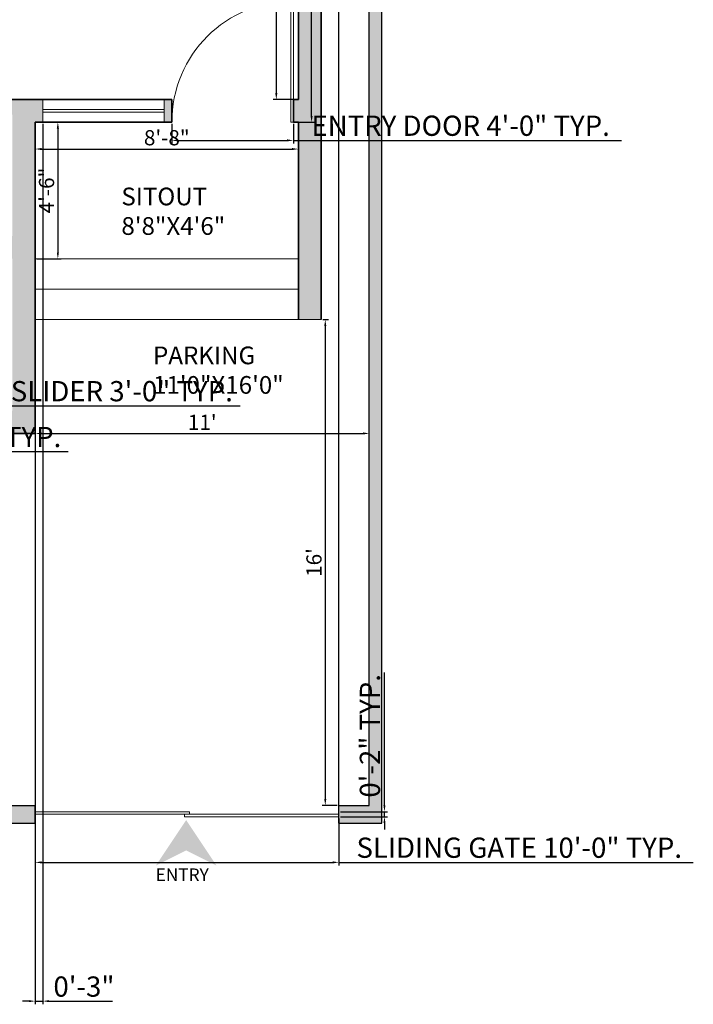
# Model space of a CAD drawing. Units: inches. Extents: x 2700 to 4052, y 1030 to 1872.
# Tile 6 of 8: x 3786 to 4052, y 1030 to 1419. Entities that reach past the tile are written whole.
import ezdxf

# ---------------------------------------------------------------- set-up
doc = ezdxf.new("R2010")
doc.units = ezdxf.units.IN
for name, color, linetype, lineweight in [('A-ANNO-DIMS', 2, 'Continuous', 13), ('A-ANNO-SYMB', 7, 'Continuous', 18), ('A-ANNO-TEXT', 7, 'Continuous', 18), ('A-AREA-IDEN', 7, 'Continuous', 18), ('A-DOOR', 4, 'Continuous', 18), ('A-FLOR-STRS', 7, 'Continuous', 18), ('A-GLAZ', 4, 'Continuous', 18), ('A-WALL', 7, 'Continuous', 35), ('A-WALL-PATT', 7, 'Continuous', 13), ('C-PROP', 7, 'Continuous', 25), ('C-SITE-GATE', 7, 'Continuous', 18)]:
    doc.layers.add(name, color=color, linetype=linetype, lineweight=lineweight)
doc.layers.add('C-SITE-PATT', color=252, linetype='Continuous', lineweight=13, true_color=0x939598)
doc.styles.get("Standard").update_dxf_attribs({"font": 'arial.ttf'})
doc.dimstyles.new('ISO-25', dxfattribs={"dimtxt": 8, "dimasz": 2.5, "dimexe": 1.25, "dimexo": 0.625, "dimtad": 1, "dimdec": 1, "dimlunit": 3, "dimtxsty": 'Standard', "dimcen": 2.5, "dimclrt": 1, "dimadec": 0, "dimazin": 0, "dimtfac": 1, "dimtdec": 1, "dimtmove": 0, "dimatfit": 3, "dimfxl": 1, "dimarcsym": 0})

# ---------------------------------------------------------------- blocks, each defined once
blk = doc.blocks.new('*D49')
at = {"layer": 'A-ANNO-DIMS', "color": 0, "lineweight": -2, "transparency": 16777216}
for p, q in [((3895.26, 1627.52), (3885.9, 1627.52)), ((3887.15, 1625.02), (3887.15, 1390.02)), ((3895.26, 1387.52), (3885.9, 1387.52))]:
    blk.add_line(p, q, dxfattribs=at)
at = {"layer": 'A-ANNO-DIMS', "color": 0, "transparency": 16777216}
for points in [[(3886.73, 1625.02), (3887.57, 1625.02), (3887.15, 1627.52)], [(3886.73, 1390.02), (3887.57, 1390.02), (3887.15, 1387.52)]]:
    blk.add_solid(points, dxfattribs=at)
at = {"layer": 'Defpoints', "color": 0, "transparency": 16777216}
for p in [(3895.88, 1627.52), (3887.15, 1387.52), (3895.88, 1387.52)]:
    blk.add_point(p, dxfattribs=at)
at = {"layer": 'A-ANNO-DIMS', "color": 0, "transparency": 16777216, "insert": (3883.46, 1507.52), "char_height": 6, "attachment_point": 5, "rotation": 90}
blk.add_mtext("20'", dxfattribs=at)
blk = doc.blocks.new('*D50')
at = {"layer": 'A-ANNO-DIMS', "color": 0, "lineweight": -2, "transparency": 16777216}
for p, q in [((3792.51, 1378.52), (3802.08, 1378.52)), ((3800.83, 1376.02), (3800.83, 1327.02)), ((3792.51, 1324.52), (3802.08, 1324.52))]:
    blk.add_line(p, q, dxfattribs=at)
at = {"layer": 'A-ANNO-DIMS', "color": 0, "transparency": 16777216}
for points in [[(3800.41, 1376.02), (3801.24, 1376.02), (3800.83, 1378.52)], [(3800.41, 1327.02), (3801.24, 1327.02), (3800.83, 1324.52)]]:
    blk.add_solid(points, dxfattribs=at)
at = {"layer": 'Defpoints', "color": 0, "transparency": 16777216}
for p in [(3791.88, 1378.52), (3791.88, 1324.52), (3800.83, 1324.52)]:
    blk.add_point(p, dxfattribs=at)
at = {"layer": 'A-ANNO-DIMS', "color": 0, "transparency": 16777216, "insert": (3797.14, 1351.52), "char_height": 6, "attachment_point": 5, "rotation": 90}
blk.add_mtext('4\'-6"', dxfattribs=at)
blk = doc.blocks.new('*D51')
at = {"layer": 'A-ANNO-DIMS', "color": 0, "lineweight": -2, "transparency": 16777216}
for p, q in [((3791.88, 1377.89), (3791.88, 1366.65)), ((3895.88, 1377.89), (3895.88, 1366.65)), ((3794.38, 1367.9), (3893.38, 1367.9))]:
    blk.add_line(p, q, dxfattribs=at)
at = {"layer": 'A-ANNO-DIMS', "color": 0, "transparency": 16777216}
for points in [[(3794.38, 1368.32), (3794.38, 1367.49), (3791.88, 1367.9)], [(3893.38, 1368.32), (3893.38, 1367.49), (3895.88, 1367.9)]]:
    blk.add_solid(points, dxfattribs=at)
at = {"layer": 'Defpoints', "color": 0, "transparency": 16777216}
for p in [(3791.88, 1378.52), (3895.88, 1378.52), (3895.88, 1367.9)]:
    blk.add_point(p, dxfattribs=at)
at = {"layer": 'A-ANNO-DIMS', "color": 0, "transparency": 16777216, "insert": (3843.88, 1371.59), "char_height": 6, "attachment_point": 5}
blk.add_mtext('8\'-8"', dxfattribs=at)
blk = doc.blocks.new('*D52')
at = {"layer": 'A-ANNO-DIMS', "color": 0, "lineweight": -2, "transparency": 16777216}
for p, q in [((3791.88, 1256.14), (3791.88, 1256.77)), ((3923.88, 1256.14), (3923.88, 1256.77)), ((3794.38, 1255.52), (3921.38, 1255.52))]:
    blk.add_line(p, q, dxfattribs=at)
at = {"layer": 'A-ANNO-DIMS', "color": 0, "transparency": 16777216}
for points in [[(3794.38, 1255.93), (3794.38, 1255.1), (3791.88, 1255.52)], [(3921.38, 1255.93), (3921.38, 1255.1), (3923.88, 1255.52)]]:
    blk.add_solid(points, dxfattribs=at)
at = {"layer": 'Defpoints', "color": 0, "transparency": 16777216}
for p in [(3791.88, 1255.52), (3923.88, 1255.52), (3923.88, 1255.52)]:
    blk.add_point(p, dxfattribs=at)
at = {"layer": 'A-ANNO-DIMS', "color": 0, "transparency": 16777216, "insert": (3857.88, 1259.15), "char_height": 6, "attachment_point": 5}
blk.add_mtext("11'", dxfattribs=at)
blk = doc.blocks.new('*D53')
at = {"layer": 'A-ANNO-DIMS', "color": 0, "lineweight": -2, "transparency": 16777216}
for p, q in [((3905.51, 1300.52), (3907.75, 1300.52)), ((3906.5, 1298.02), (3906.5, 1111.02)), ((3911.26, 1108.52), (3905.25, 1108.52))]:
    blk.add_line(p, q, dxfattribs=at)
at = {"layer": 'A-ANNO-DIMS', "color": 0, "transparency": 16777216}
for points in [[(3906.09, 1298.02), (3906.92, 1298.02), (3906.5, 1300.52)], [(3906.09, 1111.02), (3906.92, 1111.02), (3906.5, 1108.52)]]:
    blk.add_solid(points, dxfattribs=at)
at = {"layer": 'Defpoints', "color": 0, "transparency": 16777216}
for p in [(3904.88, 1300.52), (3906.5, 1108.52), (3911.88, 1108.52)]:
    blk.add_point(p, dxfattribs=at)
at = {"layer": 'A-ANNO-DIMS', "color": 0, "transparency": 16777216, "insert": (3902.81, 1204.52), "char_height": 6, "attachment_point": 5, "rotation": 90}
blk.add_mtext("16'", dxfattribs=at)
blk = doc.blocks.new('DOOR-SWING-48IN')
for p, q in [((-1, 48), (-1, 0)), ((0, 48), (0, 0)), ((0, 0), (-1, 0))]:
    blk.add_line(p, q)
blk.add_arc((0, 0), 48, 90, 180)
blk = doc.blocks.new('WINDOW-48IN')
for p, q in [((-24, -4.5), (-24, 4.5)), ((24, -4.5), (24, 4.5)), ((-24, 0.5), (24, 0.5)), ((-24, -0.5), (24, -0.5))]:
    blk.add_line(p, q)
blk = doc.blocks.new('GATE-SLIDING-120IN')
for p, q in [((0, 2), (61, 2)), ((0, 1), (120, 1)), ((59, 1), (59, 0)), ((59, 0), (120, 0)), ((61, 2), (61, 1))]:
    blk.add_line(p, q)
blk = doc.blocks.new('*D64')
at = {"layer": 'A-ANNO-DIMS', "color": 0, "lineweight": -2, "transparency": 16777216}
for p, q in [((3651.88, 1254.89), (3651.88, 1247.07)), ((3699.88, 1254.89), (3699.88, 1247.07)), ((3654.38, 1248.32), (3697.38, 1248.32)), ((3699.88, 1248.32), (3804.87, 1248.32))]:
    blk.add_line(p, q, dxfattribs=at)
at = {"layer": 'A-ANNO-DIMS', "color": 0, "transparency": 16777216}
for points in [[(3654.38, 1248.73), (3654.38, 1247.9), (3651.88, 1248.32)], [(3697.38, 1248.73), (3697.38, 1247.9), (3699.88, 1248.32)]]:
    blk.add_solid(points, dxfattribs=at)
at = {"layer": 'Defpoints', "color": 0, "transparency": 16777216}
for p in [(3651.88, 1255.52), (3699.88, 1255.52), (3699.88, 1248.32)]:
    blk.add_point(p, dxfattribs=at)
at = {"layer": 'A-ANNO-DIMS', "color": 1, "transparency": 16777216, "insert": (3753.62, 1253.08), "char_height": 8, "attachment_point": 5}
blk.add_mtext('WINDOW 4\'-0" TYP.', dxfattribs=at)
blk = doc.blocks.new('*D74')
at = {"layer": 'A-ANNO-DIMS', "color": 0, "lineweight": -2, "transparency": 16777216}
for p, q in [((3845.88, 1377.89), (3845.88, 1370.07)), ((3893.88, 1377.89), (3893.88, 1370.07)), ((3848.38, 1371.32), (3891.38, 1371.32)), ((3893.88, 1371.32), (4023.59, 1371.32))]:
    blk.add_line(p, q, dxfattribs=at)
at = {"layer": 'A-ANNO-DIMS', "color": 0, "transparency": 16777216}
for points in [[(3848.38, 1371.73), (3848.38, 1370.9), (3845.88, 1371.32)], [(3891.38, 1371.73), (3891.38, 1370.9), (3893.88, 1371.32)]]:
    blk.add_solid(points, dxfattribs=at)
at = {"layer": 'Defpoints', "color": 0, "transparency": 16777216}
for p in [(3845.88, 1378.52), (3893.88, 1378.52), (3893.88, 1371.32)]:
    blk.add_point(p, dxfattribs=at)
at = {"layer": 'A-ANNO-DIMS', "color": 1, "transparency": 16777216, "insert": (3959.99, 1376.08), "char_height": 8, "attachment_point": 5}
blk.add_mtext('ENTRY DOOR 4\'-0" TYP.', dxfattribs=at)
blk = doc.blocks.new('*D75')
at = {"layer": 'A-ANNO-DIMS', "color": 0, "lineweight": -2, "transparency": 16777216}
for p, q in [((3901.08, 1426.52), (3901.08, 1479.35)), ((3894.51, 1426.52), (3902.33, 1426.52)), ((3901.08, 1381.02), (3901.08, 1424.02)), ((3894.51, 1378.52), (3902.33, 1378.52))]:
    blk.add_line(p, q, dxfattribs=at)
at = {"layer": 'A-ANNO-DIMS', "color": 0, "transparency": 16777216}
for points in [[(3900.67, 1424.02), (3901.5, 1424.02), (3901.08, 1426.52)], [(3900.67, 1381.02), (3901.5, 1381.02), (3901.08, 1378.52)]]:
    blk.add_solid(points, dxfattribs=at)
at = {"layer": 'Defpoints', "color": 0, "transparency": 16777216}
for p in [(3893.88, 1426.52), (3901.08, 1426.52), (3893.88, 1378.52)]:
    blk.add_point(p, dxfattribs=at)
at = {"layer": 'A-ANNO-DIMS', "color": 1, "transparency": 16777216, "insert": (3896.37, 1454.19), "char_height": 8, "attachment_point": 5, "rotation": 90}
blk.add_mtext('4\'-0" TYP.', dxfattribs=at)
blk = doc.blocks.new('*D76')
at = {"layer": 'A-ANNO-DIMS', "color": 0, "lineweight": -2, "transparency": 16777216}
for p, q in [((3740.88, 1261.64), (3740.88, 1267.67)), ((3743.38, 1266.42), (3774.38, 1266.42)), ((3776.88, 1261.64), (3776.88, 1267.67)), ((3776.88, 1266.42), (3872.83, 1266.42))]:
    blk.add_line(p, q, dxfattribs=at)
at = {"layer": 'A-ANNO-DIMS', "color": 0, "transparency": 16777216}
for points in [[(3743.38, 1266.83), (3743.38, 1266), (3740.88, 1266.42)], [(3774.38, 1266.83), (3774.38, 1266), (3776.88, 1266.42)]]:
    blk.add_solid(points, dxfattribs=at)
at = {"layer": 'Defpoints', "color": 0, "transparency": 16777216}
for p in [(3776.88, 1266.42), (3740.88, 1261.02), (3776.88, 1261.02)]:
    blk.add_point(p, dxfattribs=at)
at = {"layer": 'A-ANNO-DIMS', "color": 1, "transparency": 16777216, "insert": (3826.11, 1271.18), "char_height": 8, "attachment_point": 5}
blk.add_mtext('SLIDER 3\'-0" TYP.', dxfattribs=at)
blk = doc.blocks.new('*D78')
at = {"layer": 'A-ANNO-DIMS', "color": 0, "lineweight": -2, "transparency": 16777216}
for p, q in [((3791.88, 1103.39), (3791.88, 1084.77)), ((3911.88, 1103.39), (3911.88, 1084.77)), ((3794.38, 1086.02), (3909.38, 1086.02)), ((3911.88, 1086.02), (4051.93, 1086.02))]:
    blk.add_line(p, q, dxfattribs=at)
at = {"layer": 'A-ANNO-DIMS', "color": 0, "transparency": 16777216}
for points in [[(3794.38, 1086.43), (3794.38, 1085.6), (3791.88, 1086.02)], [(3909.38, 1086.43), (3909.38, 1085.6), (3911.88, 1086.02)]]:
    blk.add_solid(points, dxfattribs=at)
at = {"layer": 'Defpoints', "color": 0, "transparency": 16777216}
for p in [(3791.88, 1104.02), (3911.88, 1104.02), (3911.88, 1086.02)]:
    blk.add_point(p, dxfattribs=at)
at = {"layer": 'A-ANNO-DIMS', "color": 1, "transparency": 16777216, "insert": (3983.15, 1090.78), "char_height": 8, "attachment_point": 5}
blk.add_mtext('SLIDING GATE 10\'-0" TYP.', dxfattribs=at)
blk = doc.blocks.new('*D79')
at = {"layer": 'A-ANNO-DIMS', "color": 0, "lineweight": -2, "transparency": 16777216}
for p, q in [((3929.88, 1108.52), (3929.88, 1161.03)), ((3912.51, 1106.02), (3931.13, 1106.02)), ((3929.88, 1104.02), (3929.88, 1106.02)), ((3912.51, 1104.02), (3931.13, 1104.02)), ((3929.88, 1101.52), (3929.88, 1099.02))]:
    blk.add_line(p, q, dxfattribs=at)
at = {"layer": 'A-ANNO-DIMS', "color": 0, "transparency": 16777216}
for points in [[(3929.47, 1108.52), (3930.3, 1108.52), (3929.88, 1106.02)], [(3929.47, 1101.52), (3930.3, 1101.52), (3929.88, 1104.02)]]:
    blk.add_solid(points, dxfattribs=at)
at = {"layer": 'Defpoints', "color": 0, "transparency": 16777216}
for p in [(3911.88, 1106.02), (3929.88, 1106.02), (3911.88, 1104.02)]:
    blk.add_point(p, dxfattribs=at)
at = {"layer": 'A-ANNO-DIMS', "color": 1, "transparency": 16777216, "insert": (3925.17, 1136.02), "char_height": 8, "attachment_point": 5, "rotation": 90}
blk.add_mtext('0\'-2" TYP.', dxfattribs=at)
blk = doc.blocks.new('*D104')
at = {"layer": 'A-ANNO-DIMS', "color": 0, "lineweight": -2, "transparency": 16777216}
for p, q in [((3911.88, 1102.14), (3911.88, 1863.37)), ((3914.38, 1862.12), (3926.38, 1862.12)), ((3928.88, 1102.14), (3928.88, 1863.37)), ((3928.88, 1862.12), (3953.15, 1862.12))]:
    blk.add_line(p, q, dxfattribs=at)
at = {"layer": 'A-ANNO-DIMS', "color": 0, "transparency": 16777216}
for points in [[(3914.38, 1862.53), (3914.38, 1861.7), (3911.88, 1862.12)], [(3926.38, 1862.53), (3926.38, 1861.7), (3928.88, 1862.12)]]:
    blk.add_solid(points, dxfattribs=at)
at = {"layer": 'Defpoints', "color": 0, "transparency": 16777216}
for p in [(3928.88, 1862.12), (3911.88, 1101.52), (3928.88, 1101.52)]:
    blk.add_point(p, dxfattribs=at)
at = {"layer": 'A-ANNO-DIMS', "color": 1, "transparency": 16777216, "insert": (3942.26, 1866.83), "char_height": 8, "attachment_point": 5}
blk.add_mtext('1\'-5"', dxfattribs=at)
blk = doc.blocks.new('*D116')
at = {"layer": 'A-ANNO-DIMS', "color": 0, "lineweight": -2, "transparency": 16777216}
for p, q in [((3791.88, 1377.89), (3791.88, 1029.93)), ((3794.88, 1377.89), (3794.88, 1029.93)), ((3789.38, 1031.18), (3786.88, 1031.18)), ((3791.88, 1031.18), (3794.88, 1031.18)), ((3797.38, 1031.18), (3822.4, 1031.18))]:
    blk.add_line(p, q, dxfattribs=at)
at = {"layer": 'A-ANNO-DIMS', "color": 0, "transparency": 16777216}
for points in [[(3789.38, 1031.6), (3789.38, 1030.77), (3791.88, 1031.18)], [(3797.38, 1031.6), (3797.38, 1030.77), (3794.88, 1031.18)]]:
    blk.add_solid(points, dxfattribs=at)
at = {"layer": 'Defpoints', "color": 0, "transparency": 16777216}
for p in [(3791.88, 1378.52), (3794.88, 1378.52), (3794.88, 1031.18)]:
    blk.add_point(p, dxfattribs=at)
at = {"layer": 'A-ANNO-DIMS', "color": 1, "transparency": 16777216, "insert": (3811.14, 1035.9), "char_height": 8, "attachment_point": 5}
blk.add_mtext('0\'-3"', dxfattribs=at)

msp = doc.modelspace()

# ---------------------------------------------------------------- hatches: boundary and pattern name
at = {"layer": 'A-ANNO-SYMB'}
h = msp.add_hatch(color=256, dxfattribs=at)
h.dxf.hatch_style = 1
h.paths.add_polyline_path([(3851.54, 1090.74), (3863.54, 1084.74), (3851.54, 1102.74), (3839.54, 1084.74)])
at = {"layer": 'A-WALL-PATT'}
h = msp.add_hatch(color=256, dxfattribs=at)
h.dxf.hatch_style = 1
h.paths.add_polyline_path([(3651.88, 1264.52), (3625.88, 1264.52), (3625.88, 1310.49), (3616.88, 1310.49), (3616.88, 1304.37), (3616.88, 1264.52), (3568.88, 1264.52), (3568.88, 1168.52), (3709.88, 1168.52), (3709.88, 1177.52), (3577.88, 1177.52), (3577.88, 1255.52), (3651.88, 1255.52)])
h.paths.add_polyline_path([(3740.88, 1264.52), (3734.88, 1264.52), (3734.88, 1324.52), (3782.88, 1324.52), (3782.88, 1264.52), (3776.88, 1264.52), (3776.88, 1255.52), (3791.88, 1255.52), (3791.88, 1378.52), (3794.88, 1378.52), (3794.88, 1387.52), (3776.88, 1387.52), (3776.88, 1381.52), (3782.88, 1381.52), (3782.88, 1333.52), (3734.88, 1333.52), (3734.88, 1381.52), (3740.88, 1381.52), (3740.88, 1387.52), (3725.88, 1387.52), (3725.88, 1264.52), (3699.88, 1264.52), (3699.88, 1255.52), (3740.88, 1255.52)])
h.paths.add_polyline_path([(3625.88, 1382.52), (3616.88, 1382.52), (3616.88, 1358.49), (3625.88, 1358.49)])
h.paths.add_polyline_path([(3845.88, 1387.52), (3842.88, 1387.52), (3842.88, 1378.52), (3845.88, 1378.52)])
h.paths.add_polyline_path([(3904.88, 1431.52), (3895.88, 1431.52), (3895.88, 1387.52), (3893.88, 1387.52), (3893.88, 1378.52), (3895.88, 1378.52), (3895.88, 1300.52), (3904.88, 1300.52)])
h.paths.add_polyline_path([(3584.49, 1565.14), (3584.49, 1604.05), (3576.25, 1604.05), (3576.25, 1565.14)], flags=9)
h.paths.add_polyline_path([(3711.56, 1565.68), (3711.56, 1611.46), (3703.32, 1611.46), (3703.32, 1565.68)], flags=9)
h.paths.add_polyline_path([(3737.75, 1697.89), (3737.75, 1743.66), (3729.51, 1743.66), (3729.51, 1697.89)], flags=9)
h.paths.add_polyline_path([(3633.29, 1800.61), (3679.06, 1800.61), (3679.06, 1808.85), (3633.29, 1808.85)], flags=9)
h.paths.add_polyline_path([(3569.7, 1361.72), (3618.67, 1361.72), (3618.67, 1388.34), (3569.7, 1388.34)], flags=9)
h.paths.add_polyline_path([(3658.81, 1318.27), (3708.12, 1318.27), (3708.12, 1344.89), (3658.81, 1344.89)], flags=9)
h.paths.add_polyline_path([(3791.11, 1507.34), (3845.25, 1507.34), (3845.25, 1533.96), (3791.11, 1533.96)], flags=9)
h.paths.add_polyline_path([(3744.61, 1774.23), (3794.63, 1774.23), (3794.63, 1800.84), (3744.61, 1800.84)], flags=9)
h.paths.add_polyline_path([(3831.1, 1774.23), (3881.17, 1774.23), (3881.17, 1800.84), (3831.1, 1800.84)], flags=9)
h.paths.add_polyline_path([(3791.11, 1664.37), (3855.09, 1664.37), (3855.09, 1690.98), (3791.11, 1690.98)], flags=9)
h.paths.add_polyline_path([(3626.06, 1747.79), (3690.04, 1747.79), (3690.04, 1774.41), (3626.06, 1774.41)], flags=9)
h.paths.add_polyline_path([(3626.06, 1590.97), (3690.04, 1590.97), (3690.04, 1617.58), (3626.06, 1617.58)], flags=9)
h.paths.add_polyline_path([(3616.71, 1447.4), (3665.68, 1447.4), (3665.68, 1474.01), (3616.71, 1474.01)], flags=9)
at = {"layer": 'C-SITE-PATT'}
h = msp.add_hatch(color=256, dxfattribs=at)
h.dxf.hatch_style = 1
h.paths.add_polyline_path([(3573.88, 1821.52), (3568.88, 1821.52), (3568.88, 1423.52), (3573.88, 1423.52)])
h.paths.add_polyline_path([(3791.88, 1108.52), (3573.88, 1108.52), (3573.88, 1168.52), (3568.88, 1168.52), (3568.88, 1101.52), (3791.88, 1101.52)])
h.paths.add_polyline_path([(3928.88, 1821.52), (3923.88, 1821.52), (3923.88, 1108.52), (3911.88, 1108.52), (3911.88, 1101.52), (3928.88, 1101.52)])

# ---------------------------------------------------------------- linework, layer by layer
at = {"layer": 'A-FLOR-STRS'}
for p, q in [((3895.88, 1324.52), (3791.88, 1324.52)), ((3895.88, 1312.52), (3791.88, 1312.52)), ((3904.88, 1300.52), (3791.88, 1300.52))]:
    msp.add_line(p, q, dxfattribs=at)
at = {"layer": 'A-WALL'}
for p, q in [((3904.88, 1300.52), (3904.88, 1821.52)), ((3895.88, 1387.52), (3895.88, 1627.52)), ((3845.88, 1387.52), (3776.88, 1387.52)), ((3845.88, 1378.52), (3845.88, 1387.52)), ((3895.88, 1387.52), (3893.88, 1387.52)), ((3893.88, 1378.52), (3893.88, 1387.52)), ((3845.88, 1378.52), (3791.88, 1378.52)), ((3791.88, 1255.52), (3791.88, 1378.52)), ((3895.88, 1378.52), (3893.88, 1378.52)), ((3895.88, 1300.52), (3895.88, 1378.52)), ((3791.88, 1255.52), (3776.88, 1255.52))]:
    msp.add_line(p, q, dxfattribs=at)
at = {"layer": 'C-PROP'}
for p, q in [((3923.88, 1108.52), (3923.88, 1821.52)), ((3573.88, 1108.52), (3791.88, 1108.52)), ((3791.88, 1101.52), (3791.88, 1108.52)), ((3911.88, 1108.52), (3923.88, 1108.52)), ((3911.88, 1101.52), (3911.88, 1108.52))]:
    msp.add_line(p, q, dxfattribs=at)
msp.add_lwpolyline([(3911.88, 1101.52), (3928.88, 1101.52), (3928.88, 1821.52), (3568.88, 1821.52), (3568.88, 1101.52), (3791.88, 1101.52)], dxfattribs=at)

# ---------------------------------------------------------------- block references
at = {"layer": 'A-DOOR'}
msp.add_blockref('DOOR-SWING-48IN', (3893.88, 1378.52), dxfattribs=at)
at = {"layer": 'A-GLAZ', "rotation": 180}
msp.add_blockref('WINDOW-48IN', (3818.88, 1383.02), dxfattribs=at)
at = {"layer": 'C-SITE-GATE'}
msp.add_blockref('GATE-SLIDING-120IN', (3791.88, 1104.02), dxfattribs=at)

# ---------------------------------------------------------------- texts
at = {"layer": 'A-ANNO-TEXT', "insert": (3839.47, 1083.62), "char_height": 5, "attachment_point": 1}
msp.add_mtext_dynamic_manual_height_columns('{\\fTimes New Roman|b0|i0|c0|p18;ENTRY}', width=196.2607, gutter_width=12.5, heights=[0], dxfattribs=at)
at = {"layer": 'A-AREA-IDEN', "char_height": 7, "attachment_point": 1}
for s, insert in [('{\\fTimes New Roman|b0|i0|c0|p18;SITOUT\\P8\'8"X4\'6"}', (3825.93, 1352.66)), ('{\\fTimes New Roman|b0|i0|c0|p18;PARKING\\P11\'0"X16\'0"}', (3838.44, 1289.86))]:
    msp.add_mtext_dynamic_manual_height_columns(s, width=61.0557, gutter_width=12.5, heights=[0], dxfattribs=dict(at, insert=insert))

# ---------------------------------------------------------------- dimensions: what is measured, and where the dimension line sits
at = {"layer": 'A-ANNO-DIMS'}
for base, p1, p2, override, picture, middle in [((3928.88, 1862.12), (3911.88, 1101.52), (3928.88, 1101.52), {"dimdec": 1, "dimlfac": 1, "dimrnd": 0, "dimzin": 1, "dimdsep": 46, "dimlunit": 4, "dimfrac": 2}, '*D104', (3942.26, 1866.83)), ((3794.88, 1031.18), (3791.88, 1378.52), (3794.88, 1378.52), {"dimdec": 1, "dimlfac": 1, "dimrnd": 0, "dimzin": 1, "dimdsep": 46, "dimlunit": 4, "dimfrac": 2}, '*D116', (3811.14, 1035.9)), ((3895.88, 1367.9), (3791.88, 1378.52), (3895.88, 1378.52), {"dimtxt": 6, "dimclrd": 0, "dimclre": 0, "dimclrt": 0}, '*D51', (3843.88, 1371.59)), ((3923.88, 1255.52), (3791.88, 1255.52), (3923.88, 1255.52), {"dimtxt": 6, "dimclrd": 0, "dimclre": 0, "dimclrt": 0}, '*D52', (3857.88, 1259.15))]:
    dim = msp.add_linear_dim(base=base, p1=p1, p2=p2, dimstyle='ISO-25', override=override, dxfattribs=at)
    dim.commit()
    dim.dimension.update_dxf_attribs({"geometry": picture, "text_midpoint": middle})
for base, p1, p2, picture, middle in [((3887.15, 1387.52), (3895.88, 1627.52), (3895.88, 1387.52), '*D49', (3883.46, 1507.52)), ((3800.83, 1324.52), (3791.88, 1378.52), (3791.88, 1324.52), '*D50', (3797.14, 1351.52)), ((3906.5, 1108.52), (3904.88, 1300.52), (3911.88, 1108.52), '*D53', (3902.81, 1204.52))]:
    dim = msp.add_linear_dim(base=base, p1=p1, p2=p2, angle=90, dimstyle='ISO-25', override={"dimtxt": 6, "dimclrd": 0, "dimclre": 0, "dimclrt": 0}, dxfattribs=at)
    dim.commit()
    dim.dimension.update_dxf_attribs({"geometry": picture, "text_midpoint": middle})
for base, p1, p2, picture, middle in [((3901.08, 1426.52), (3893.88, 1378.52), (3893.88, 1426.52), '*D75', (3896.37, 1454.19)), ((3929.88, 1106.02), (3911.88, 1104.02), (3911.88, 1106.02), '*D79', (3925.17, 1136.02))]:
    dim = msp.add_linear_dim(base=base, p1=p1, p2=p2, angle=90, text='<> TYP.', dimstyle='ISO-25', override={"dimdec": 1, "dimlfac": 1, "dimrnd": 0, "dimzin": 1, "dimdsep": 46, "dimlunit": 4, "dimfrac": 2}, dxfattribs=at)
    dim.commit()
    dim.dimension.update_dxf_attribs({"geometry": picture, "text_midpoint": middle})
for base, p1, p2, text, picture, middle in [((3893.88, 1371.32), (3845.88, 1378.52), (3893.88, 1378.52), 'ENTRY DOOR <> TYP.', '*D74', (3959.99, 1376.08)), ((3776.88, 1266.42), (3740.88, 1261.02), (3776.88, 1261.02), 'SLIDER <> TYP.', '*D76', (3826.11, 1271.18)), ((3699.88, 1248.32), (3651.88, 1255.52), (3699.88, 1255.52), 'WINDOW <> TYP.', '*D64', (3753.62, 1253.08)), ((3911.88, 1086.02), (3791.88, 1104.02), (3911.88, 1104.02), 'SLIDING GATE <> TYP.', '*D78', (3983.15, 1090.78))]:
    dim = msp.add_linear_dim(base=base, p1=p1, p2=p2, text=text, dimstyle='ISO-25', override={"dimdec": 1, "dimlfac": 1, "dimrnd": 0, "dimzin": 1, "dimdsep": 46, "dimlunit": 4, "dimfrac": 2}, dxfattribs=at)
    dim.commit()
    dim.dimension.update_dxf_attribs({"geometry": picture, "text_midpoint": middle})

doc.saveas('drawing.dxf')
